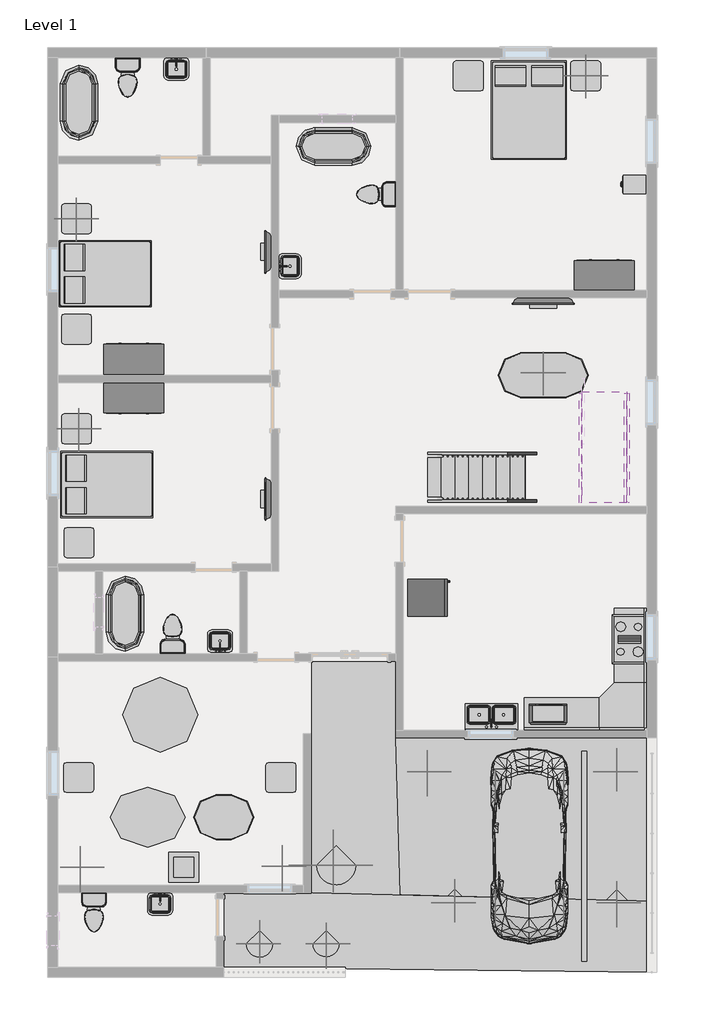
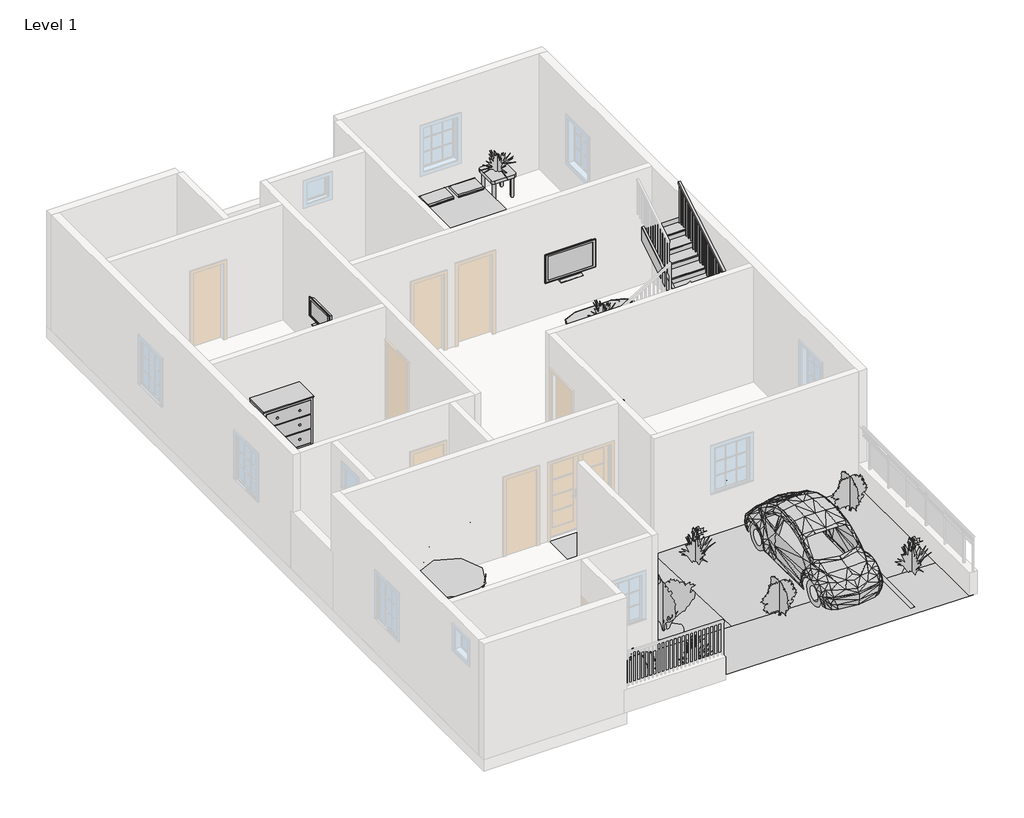
# One storey, part 3 of 3: 24 furniture elements, 16 flow terminals, 13 geographic elements, 8 proxies, 4 members, 2 stair flights, 1 railing.
# Revit data of these elements (continued)
# Materials (continued)
#   "Porcelain, Linen": class "Ceramic", colour RGB 249 239 230, transparency 0, Description = "Porcelain, linen", Cost = 0
#   "Laminate, Linen, Matte": class "Plastic", colour RGB 249 239 230, transparency 0, Description = "Plastic Laminate - Linen, Matte", Cost = 0
#   "Porcelain, Ivory": class "Ceramic", colour RGB 247 247 239, transparency 0, Description = "Porcelain, ivory", Cost = 0
#   "Birch": class "Wood", colour RGB 224 178 126, transparency 0, Description = "Betula Alleghaniensis", Cost = 0
#   "Linen, White": class "Textile", colour RGB 247 247 239, transparency 0, Description = "Linen, white", Cost = 0
#   "Laminate - Ivory, Glossy": colour RGB 247 247 239, transparency 0
#   "Cherry": class "Wood", colour RGB 226 177 128, transparency 0, Description = "Prunus Serotina", Cost = 0
#   "Glass - Clear, Grey": class "Glass", colour RGB 252 255 255, transparency 0.64
#   "Pine": class "Wood", colour RGB 223 192 134, transparency 0, Description = "Pinus Echinata", Cost = 0
#   "Textile - Light Gray": class "Fabric", colour RGB 204 204 204, transparency 0
#   "Glass": class "Glass", colour RGB 0 128 192, transparency 0.75, Description = "Soda Lime Glass", Cost = 0
#   "Parking Stripe": class "Paint", colour RGB 250 250 91, transparency 0
#   "TV - Black": colour RGB 49 49 49, transparency 0
#   "TV - Glass": colour RGB 157 157 157, transparency 0.9
#   "TV - Screen": colour RGB 0 0 0, transparency 0
